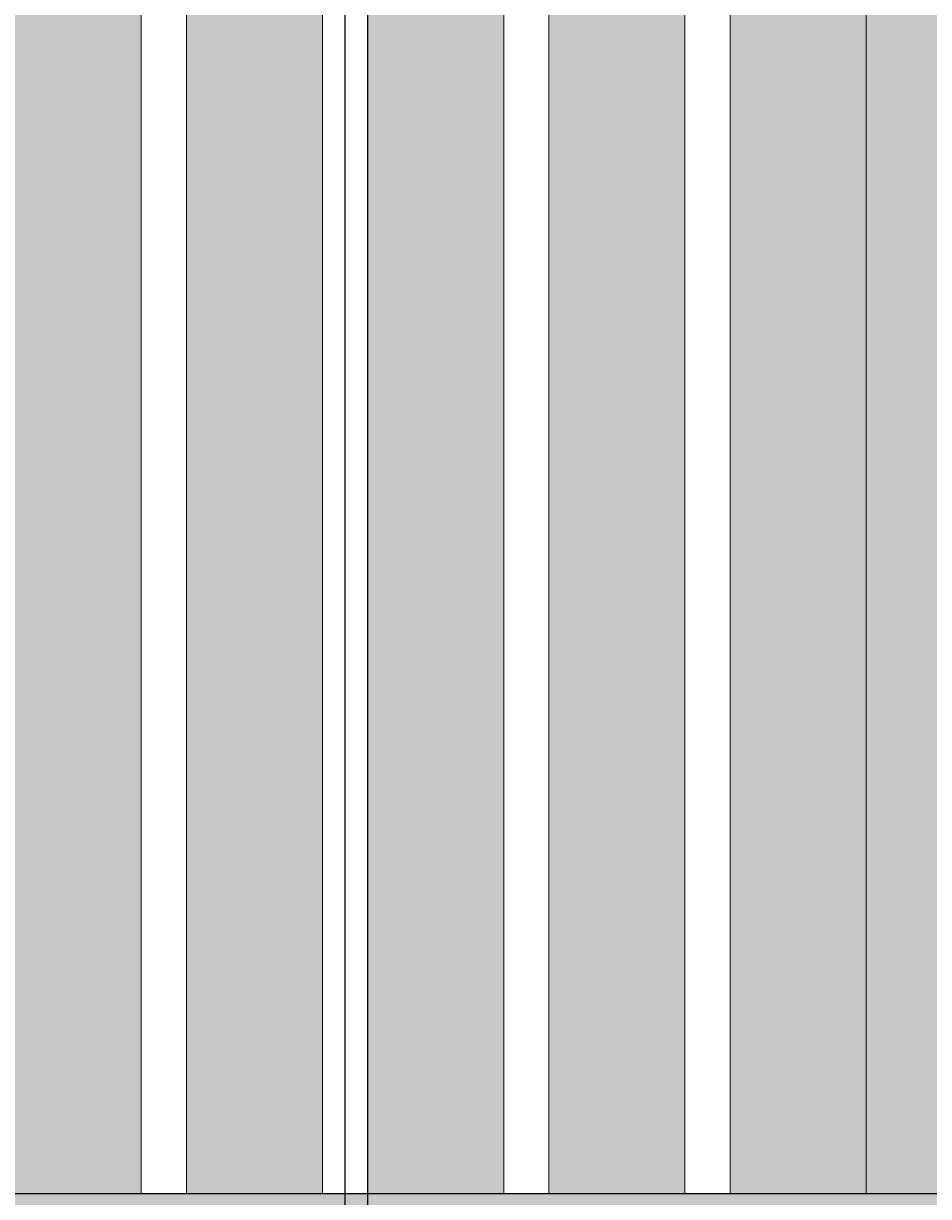
# Model space of a CAD drawing. Units: inches. Extents: x 4508 to 4723, y 847 to 1020.
# Tile 10 of 32: x 4570 to 4590, y 905 to 931. Entities that reach past the tile are written whole.
import ezdxf

# ---------------------------------------------------------------- set-up
doc = ezdxf.new("R2010")
doc.units = ezdxf.units.IN
for name, color, linetype, lineweight in [('A-ANNO-DIMS', 2, 'Continuous', 18), ('A-FURN', 8, 'Continuous', 25), ('A-WALL-FINS', 30, 'Continuous', 18), ('A-WALL-PATT', 254, 'Continuous', 13)]:
    doc.layers.add(name, color=color, linetype=linetype, lineweight=lineweight)
doc.styles.get("Standard").update_dxf_attribs({"font": 'arial.ttf'})
doc.dimstyles.get("Standard").update_dxf_attribs({"dimtxt": 0.18, "dimasz": 0.18, "dimexe": 0.18, "dimexo": 0.0625, "dimgap": 0.09, "dimtad": 0, "dimtih": 1, "dimtoh": 1, "dimdec": 4, "dimzin": 0, "dimdsep": 46, "dimtxsty": 'Standard', "dimcen": 0.09, "dimadec": 0, "dimazin": 0, "dimtfac": 1, "dimtdec": 4, "dimtofl": 0, "dimtmove": 0, "dimatfit": 3, "dimfxl": 1, "dimtolj": 1, "dimtzin": 0, "dimarcsym": 0})

# ---------------------------------------------------------------- blocks, each defined once
blk = doc.blocks.new('*D27')
at = {"layer": 'A-ANNO-DIMS', "color": 0, "lineweight": -2, "transparency": 16777216}
for p, q in [((4550.994, 903.809), (4550.994, 1002.877)), ((4577.494, 903.809), (4577.494, 1002.877)), ((4551.174, 1002.697), (4563.918, 1002.697)), ((4577.314, 1002.697), (4564.57, 1002.697))]:
    blk.add_line(p, q, dxfattribs=at)
at = {"layer": 'A-ANNO-DIMS', "color": 0, "lineweight": 9, "transparency": 16777216}
for points in [[(4551.174, 1002.727), (4551.174, 1002.667), (4550.994, 1002.697)], [(4577.314, 1002.727), (4577.314, 1002.667), (4577.494, 1002.697)]]:
    blk.add_solid(points, dxfattribs=at)
at = {"layer": 'Defpoints', "color": 0, "lineweight": 9, "transparency": 16777216}
for p in [(4577.494, 1002.697), (4550.994, 903.747), (4577.494, 903.747)]:
    blk.add_point(p, dxfattribs=at)
at = {"layer": 'A-ANNO-DIMS', "color": 0, "transparency": 16777216, "insert": (4564.244, 1002.697), "char_height": 0.18, "attachment_point": 5}
blk.add_mtext('\\A1;26.5', dxfattribs=at)
blk = doc.blocks.new('*D28')
at = {"layer": 'A-ANNO-DIMS', "color": 0, "lineweight": -2, "transparency": 16777216}
for p, q in [((4577.494, 903.809), (4577.494, 1002.877)), ((4577.994, 903.809), (4577.994, 1002.877)), ((4577.314, 1002.697), (4577.134, 1002.697)), ((4578.174, 1002.697), (4578.354, 1002.697))]:
    blk.add_line(p, q, dxfattribs=at)
at = {"layer": 'A-ANNO-DIMS', "color": 0, "lineweight": 9, "transparency": 16777216}
for points in [[(4577.314, 1002.727), (4577.314, 1002.667), (4577.494, 1002.697)], [(4578.174, 1002.727), (4578.174, 1002.667), (4577.994, 1002.697)]]:
    blk.add_solid(points, dxfattribs=at)
at = {"layer": 'Defpoints', "color": 0, "lineweight": 9, "transparency": 16777216}
for p in [(4577.994, 1002.697), (4577.494, 903.747), (4577.994, 903.747)]:
    blk.add_point(p, dxfattribs=at)
at = {"layer": 'A-ANNO-DIMS', "color": 0, "transparency": 16777216, "insert": (4578.608, 1002.697), "char_height": 0.18, "attachment_point": 5}
blk.add_mtext('\\A1;0.5', dxfattribs=at)
blk = doc.blocks.new('*D29')
at = {"layer": 'A-ANNO-DIMS', "color": 0, "lineweight": -2, "transparency": 16777216}
for p, q in [((4577.994, 903.809), (4577.994, 1002.877)), ((4603.994, 903.809), (4603.994, 1002.877)), ((4578.174, 1002.697), (4590.773, 1002.697)), ((4603.814, 1002.697), (4591.214, 1002.697))]:
    blk.add_line(p, q, dxfattribs=at)
at = {"layer": 'A-ANNO-DIMS', "color": 0, "lineweight": 9, "transparency": 16777216}
for points in [[(4578.174, 1002.727), (4578.174, 1002.667), (4577.994, 1002.697)], [(4603.814, 1002.727), (4603.814, 1002.667), (4603.994, 1002.697)]]:
    blk.add_solid(points, dxfattribs=at)
at = {"layer": 'Defpoints', "color": 0, "lineweight": 9, "transparency": 16777216}
for p in [(4603.994, 1002.697), (4577.994, 903.747), (4603.994, 903.747)]:
    blk.add_point(p, dxfattribs=at)
at = {"layer": 'A-ANNO-DIMS', "color": 0, "transparency": 16777216, "insert": (4590.994, 1002.697), "char_height": 0.18, "attachment_point": 5}
blk.add_mtext('\\A1;26', dxfattribs=at)

msp = doc.modelspace()

# ---------------------------------------------------------------- hatches: boundary and pattern name
at = {"layer": 'A-WALL-PATT', "transparency": 33554681}
h = msp.add_hatch(color=256, dxfattribs=at)
h.dxf.hatch_style = 1
h.paths.add_polyline_path([(4552.9938, 994.7469), (4549.9938, 994.7469), (4549.9938, 904.7469), (4552.9938, 904.7469)])
h.paths.add_polyline_path([(4556.9938, 994.7469), (4553.9938, 994.7469), (4553.9938, 904.7469), (4556.9938, 904.7469)])
h.paths.add_polyline_path([(4560.9938, 994.7469), (4557.9938, 994.7469), (4557.9938, 904.7469), (4560.9938, 904.7469)])
h.paths.add_polyline_path([(4564.9938, 994.7469), (4561.9938, 994.7469), (4561.9938, 904.7469), (4564.9938, 904.7469)])
h.paths.add_polyline_path([(4568.9938, 994.7469), (4565.9938, 994.7469), (4565.9938, 904.7469), (4568.9938, 904.7469)])
h.paths.add_polyline_path([(4572.9938, 994.7469), (4569.9938, 994.7469), (4569.9938, 904.7469), (4572.9938, 904.7469)])
h.paths.add_polyline_path([(4576.9938, 994.7469), (4573.9938, 994.7469), (4573.9938, 904.7469), (4576.9938, 904.7469)])
h.paths.add_polyline_path([(4580.9938, 994.7469), (4577.9938, 994.7469), (4577.9938, 904.7469), (4580.9938, 904.7469)])
h.paths.add_polyline_path([(4584.9938, 994.7469), (4581.9938, 994.7469), (4581.9938, 904.7469), (4584.9938, 904.7469)])
at = {"layer": 'A-WALL-PATT', "transparency": 33554508}
h = msp.add_hatch(color=256, dxfattribs=at)
h.dxf.hatch_style = 1
h.paths.add_polyline_path([(4661.6706, 954.043, -0.3739004), (4658.5765, 957.6021, -1), (4665.7646, 957.6021, -0.3739004), (4662.6706, 954.043), (4662.6706, 944.4021, -0.2114781), (4670.3062, 945.0869), (4670.3062, 968.0592, -0.4632086), (4663.3246, 973.9783, -0.4632086), (4670.3062, 979.8975), (4670.3062, 994.7469), (4588.9938, 994.7469), (4588.9938, 904.7469), (4657.9938, 904.7469), (4657.9938, 886.7469), (4549.9938, 886.7469), (4549.9938, 878.7469), (4693.9938, 878.7469), (4693.9938, 994.7469), (4671.8062, 994.7469), (4671.8062, 979.4411, -0.2941682), (4675.3246, 973.9783, -0.2941682), (4671.8062, 968.5156), (4671.8062, 944.4278, -0.2741114), (4676.7298, 936.1217, -0.2741114), (4671.8062, 927.8155), (4671.8062, 907.6998, -0.3779645), (4677.0562, 901.7469, -0.3779645), (4671.8062, 895.7939), (4671.8062, 883.7469), (4670.3062, 883.7469), (4670.3062, 895.7939, -0.3779645), (4665.0562, 901.7469, -0.3779645), (4670.3062, 907.6998), (4670.3062, 927.1564, -0.2114781), (4662.6706, 927.8412), (4662.6706, 918.2003, -0.3739004), (4665.7646, 914.6412, -1), (4658.5765, 914.6412, -0.3739004), (4661.6706, 918.2003), (4661.6706, 928.4807, -0.2391825), (4657.7936, 936.1217, -0.2391825), (4661.6706, 943.7626)])
at = {"layer": 'A-WALL-PATT', "transparency": 33554681}
h = msp.add_hatch(color=256, dxfattribs=at)
h.dxf.hatch_style = 1
h.paths.add_polyline_path([(4588.9938, 994.7469), (4585.9938, 994.7469), (4585.9938, 904.7469), (4588.9938, 904.7469)])
h = msp.add_hatch(color=256, dxfattribs=at)
h.dxf.hatch_style = 1
h.paths.add_polyline_path([(4577.4938, 903.7469), (4550.9938, 903.7469), (4550.9938, 887.7469), (4577.4938, 887.7469)], flags=0)
h.paths.add_polyline_path([(4603.9938, 903.7469), (4577.9938, 903.7469), (4577.9938, 887.7469), (4603.9938, 887.7469)], flags=0)
h.paths.add_polyline_path([(4656.9938, 903.7469), (4630.9938, 903.7469), (4630.9938, 887.7469), (4656.9938, 887.7469)], flags=0)
h.paths.add_polyline_path([(4657.9938, 904.7469), (4549.9938, 904.7469), (4549.9938, 886.7469), (4657.9938, 886.7469)])
h.paths.add_polyline_path([(4656.9938, 903.7469), (4656.9938, 887.7469), (4550.9938, 887.7469), (4550.9938, 903.7469)], flags=16)

# ---------------------------------------------------------------- linework, layer by layer
at = {"layer": 'A-FURN'}
msp.add_lwpolyline([(4657.9938, 886.7469), (4549.9938, 886.7469), (4549.9938, 904.7469), (4657.9938, 904.7469)], close=True, dxfattribs=at)
at = {"layer": 'A-WALL-FINS'}
for p, q in [((4572.9938, 904.7469), (4572.9938, 994.7469)), ((4573.9938, 904.7469), (4573.9938, 994.7469)), ((4576.9938, 904.7469), (4576.9938, 994.7469)), ((4577.9938, 904.7469), (4577.9938, 994.7469)), ((4580.9938, 904.7469), (4580.9938, 994.7469)), ((4581.9938, 904.7469), (4581.9938, 994.7469)), ((4584.9938, 904.7469), (4584.9938, 994.7469)), ((4585.9938, 904.7469), (4585.9938, 994.7469)), ((4588.9938, 904.7469), (4588.9938, 994.7469))]:
    msp.add_line(p, q, dxfattribs=at)

# ---------------------------------------------------------------- dimensions: what is measured, and where the dimension line sits
at = {"layer": 'A-ANNO-DIMS'}
for base, p1, p2, override, picture, middle in [((4577.4938, 1002.6969), (4550.9938, 903.7469), (4577.4938, 903.7469), {"dimdec": 1, "dimlfac": 1, "dimrnd": 0, "dimzin": 0, "dimdsep": 46, "dimlunit": 2}, '*D27', (4564.2438, 1002.6969)), ((4577.9938, 1002.6969), (4577.4938, 903.7469), (4577.9938, 903.7469), {"dimdec": 1, "dimlfac": 1, "dimrnd": 0, "dimzin": 0, "dimdsep": 46, "dimlunit": 2}, '*D28', (4578.6083, 1002.6969)), ((4603.9938, 1002.6969), (4577.9938, 903.7469), (4603.9938, 903.7469), {"dimdec": 0, "dimlfac": 1, "dimrnd": 0, "dimzin": 0, "dimdsep": 46, "dimlunit": 2}, '*D29', (4590.9938, 1002.6969))]:
    dim = msp.add_linear_dim(base=base, p1=p1, p2=p2, dimstyle='Standard', override=override, dxfattribs=at)
    dim.commit()
    dim.dimension.update_dxf_attribs({"geometry": picture, "text_midpoint": middle})

doc.saveas('drawing.dxf')
